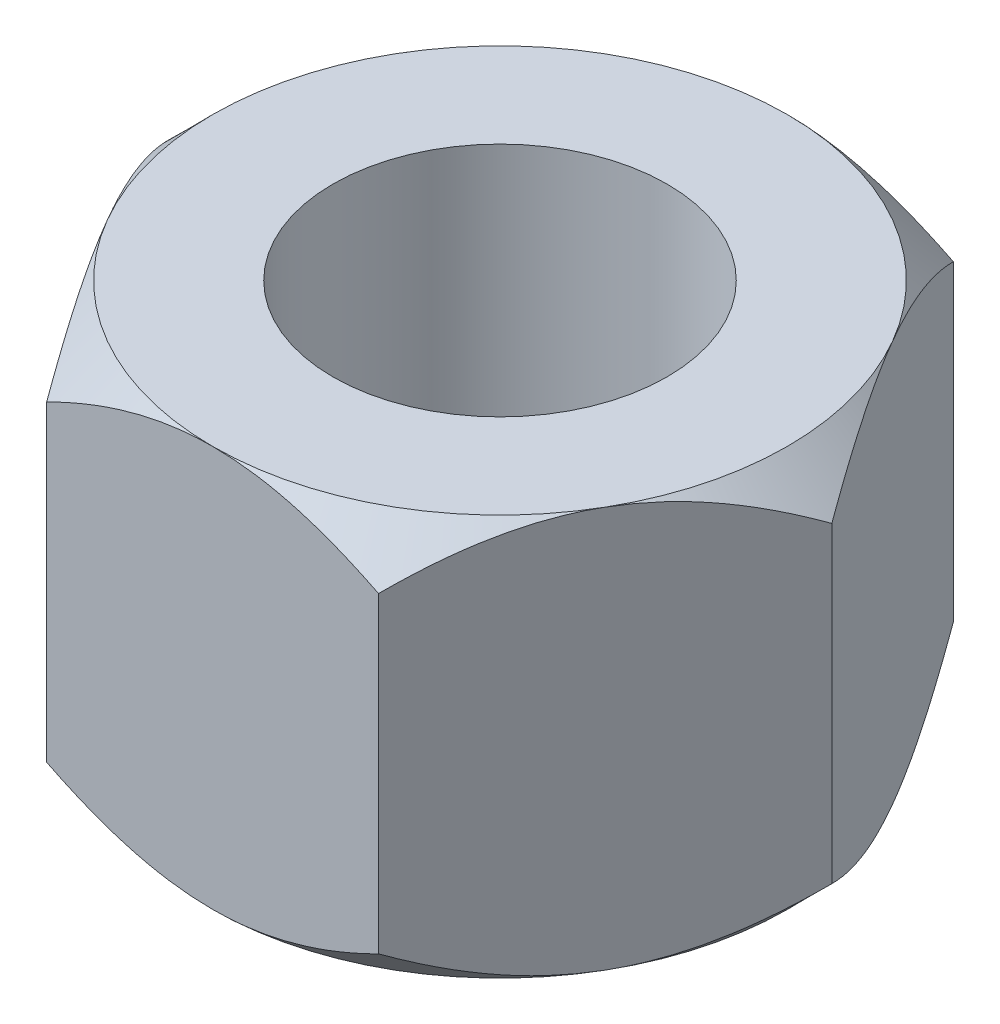
SolidWorks part; units mm, degrees
material "Plain Carbon Steel"
ref_plane "Front Plane" through (0, 0, 0) normal (0, 0, 1) x (1, 0, 0)
ref_plane "Top Plane" through (0, 0, 0) normal (0, 1, 0) x (1, 0, 0)
ref_plane "Right Plane" through (0, 0, 0) normal (1, 0, 0) x (0, 0, -1)
sketch "Hex Profile 4.3AF Sketch" plane through (0, 0, 0) normal (0, 1, 0) x (1, 0, 0)
  line L1 (1.2413, -2.15) -> (2.4826, 0)
  line L2 (2.4826, 0) -> (1.2413, 2.15)
  line L3 (1.2413, 2.15) -> (-1.2413, 2.15)
  line L4 (-1.2413, 2.15) -> (-2.4826, 0)
  line L5 (-2.4826, 0) -> (-1.2413, -2.15)
  line L6 (-1.2413, -2.15) -> (1.2413, -2.15)
  circle A0 centre (0, 0) radius 2.15 construction
  dimension "D1" = 4.3
extrude "Hex Body 3mm" add sketch "Hex Profile 4.3AF Sketch" along normal blind 3
sketch "Face Chamfer A Sketch" plane through (0, 3, 0) normal (0, 1, 0) x (1, 0, 0)
  line L0 (-1.2413, -2.15) -> (1.2413, -2.15) construction
  circle A0 centre (0, 0) radius 2.15
extrude "Face Chamfer A 45deg" cut sketch "Face Chamfer A Sketch" against normal blind 3 draft 45 flip side to cut
sketch "Face Chamfer B Sketch" plane through (0, 0, 0) normal (0, -1, 0) x (1, 0, 0)
  line L0 (1.2413, -2.15) -> (-1.2413, -2.15) construction
  circle A0 centre (0, 0) radius 2.15
extrude "Face Chamfer B 45deg" cut sketch "Face Chamfer B Sketch" against normal blind 3 draft 45 flip side to cut
sketch "Bore Ø2.5 Sketch" plane through (0, 0, 0) normal (0, -1, 0) x (1, 0, 0)
  circle A0 centre (0, 0) radius 1.25
  dimension "D1" = 2.5
extrude "Through Bore Ø2.5" cut sketch "Bore Ø2.5 Sketch" against normal blind 23
